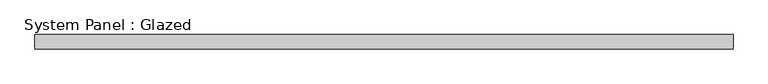
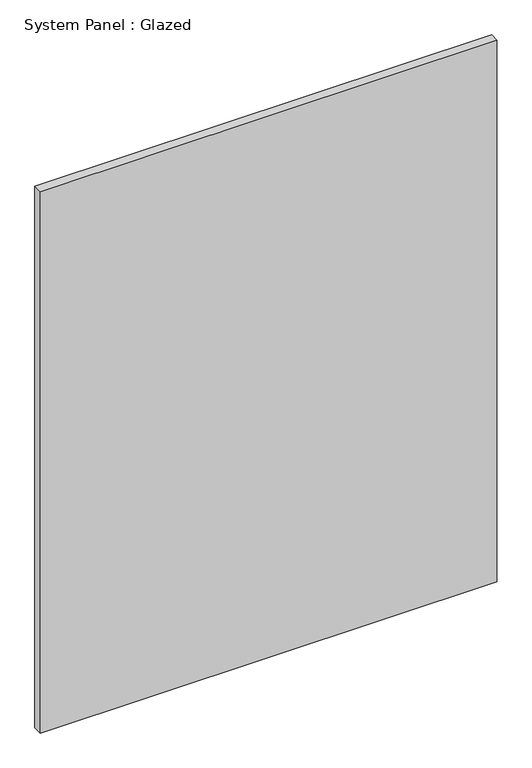
"""IFC4 building model written with IfcOpenShell, lengths in millimetres: plate geometry, System Panel : Glazed."""

from ifc_helpers import new_model, si_unit, origin, origin_with_axes, place, context, project, spatial, polyline, outline, extrude, source, transform, mapped, element, save


def system_panel_glazed_a16c717b(model_context):
    return source(origin(), model_context, "Body", "SweptSolid", [
        extrude(outline(polyline([(612.3937105, 19.05), (-612.3937105, 19.05), (-612.3937105, 44.45), (612.3937105, 44.45), (612.3937105, 19.05)])), origin_with_axes(), (0.0, 0.0, 1.0), 1535.7829369),
    ])


if __name__ == "__main__":
    model = new_model("IFC4")
    model_context = context("Model", 3, world=origin())
    ifc_project = project(units=[si_unit("LENGTHUNIT", "METRE", prefix="MILLI")], contexts=[model_context])
    site = spatial("IfcSite", under=ifc_project)
    building = spatial("IfcBuilding", under=site)
    placement = place(None, origin())
    system_panel_glazed_shape = system_panel_glazed_a16c717b(model_context)
    element("IfcPlate", 1, ObjectType="System Panel : Glazed", at=placement, inside=building, context=model_context, shape_type="MappedRepresentation", body=[
        mapped(system_panel_glazed_shape, transform((0.0, 0.0, 0.0), x_axis=(1.0, 0.0, 0.0), y_axis=(0.0, 1.0, 0.0), z_axis=(0.0, 0.0, 1.0))),
    ])
    save(model, "model.ifc")

# Revit data of these elements
# Type "System Panel : Glazed"
#   Construction Type Id = "GSP4R"
#   Analytic Construction = "1/8 in Pilkington single glazing"
#   Visual Light Transmittance = 0.9
#   Solar Heat Gain Coefficient = 0.86
#   Heat Transfer Coefficient (U) = 1.18115 BTU/(h·ft²·°F)
#   Define Thermal Properties by = 1
# Element 1 (IfcPlate, "System Panel : Glazed")
#   Materials on its faces: "Glass"
# Materials
#   "Glass": class "Glass", colour RGB 0 128 192, transparency 0.75, Description = "Soda Lime Glass", Cost = 0
